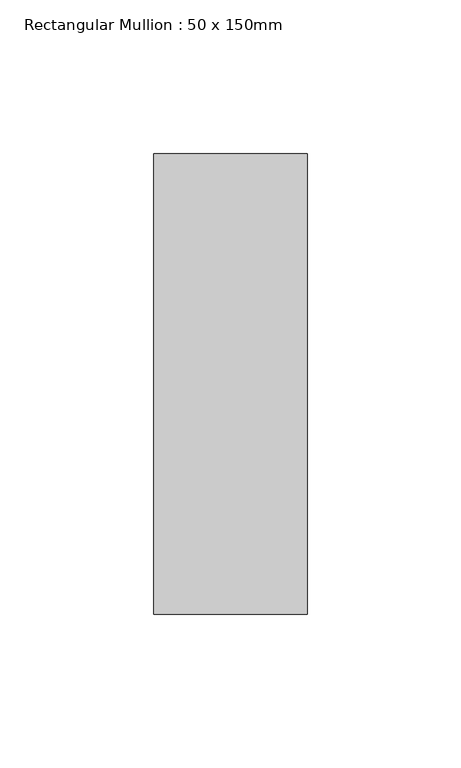
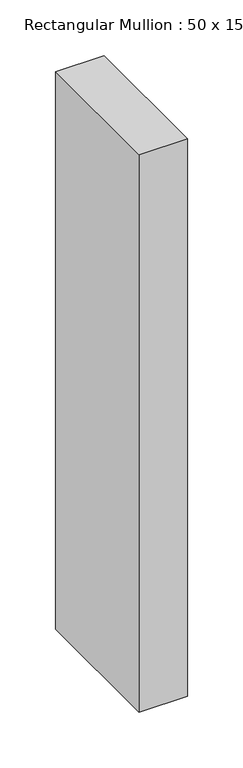
"""IFC4 building model written with IfcOpenShell, lengths in millimetres: member geometry, Rectangular Mullion : 50 x 150mm."""

from ifc_helpers import new_model, si_unit, frame, origin, place, context, project, spatial, polyline, outline, extrude, source, transform, mapped, element, save


def rectangular_mullion_50_x_150mm_c6835c94(model_context):
    return source(origin(), model_context, "Body", "SweptSolid", [
        extrude(outline(polyline([(0.0, 75.0), (0.0, -75.0), (-50.0, -75.0), (-50.0, 75.0), (0.0, 75.0)])), frame((0.0, 0.0, -610.0), z_axis=(0.0, 0.0, 1.0), x_axis=(1.0, 0.0, 0.0)), (0.0, 0.0, 1.0), 610.0),
    ])


if __name__ == "__main__":
    model = new_model("IFC4")
    model_context = context("Model", 3, world=origin())
    ifc_project = project(units=[si_unit("LENGTHUNIT", "METRE", prefix="MILLI")], contexts=[model_context])
    site = spatial("IfcSite", under=ifc_project)
    building = spatial("IfcBuilding", under=site)
    placement = place(None, origin())
    rectangular_mullion_50_x_150mm_shape = rectangular_mullion_50_x_150mm_c6835c94(model_context)
    element("IfcMember", 1, ObjectType="Rectangular Mullion : 50 x 150mm", at=placement, inside=building, context=model_context, shape_type="MappedRepresentation", body=[
        mapped(rectangular_mullion_50_x_150mm_shape, transform((0.0, 0.0, 0.0), x_axis=(1.0, 0.0, 0.0), y_axis=(0.0, 1.0, 0.0), z_axis=(0.0, 0.0, 1.0))),
    ])
    save(model, "model.ifc")

# Revit data of these elements
# Type "Rectangular Mullion : 50 x 150mm"
#   built-in parameter 1007304 = 0.492126 (stored number, unit not read)
#   built-in parameter 1007301 = 0.082021 (stored number, unit not read)
#   built-in parameter 1007300 = 0.082021 (stored number, unit not read)
# Element 1 (IfcMember, "Rectangular Mullion : 50 x 150mm")
#   Materials on its faces: "Aluminium"
# Materials
#   "Aluminium": class "Metal", colour RGB 247 247 247, transparency 0, Description = "Aluminium 6061", Cost = 0
